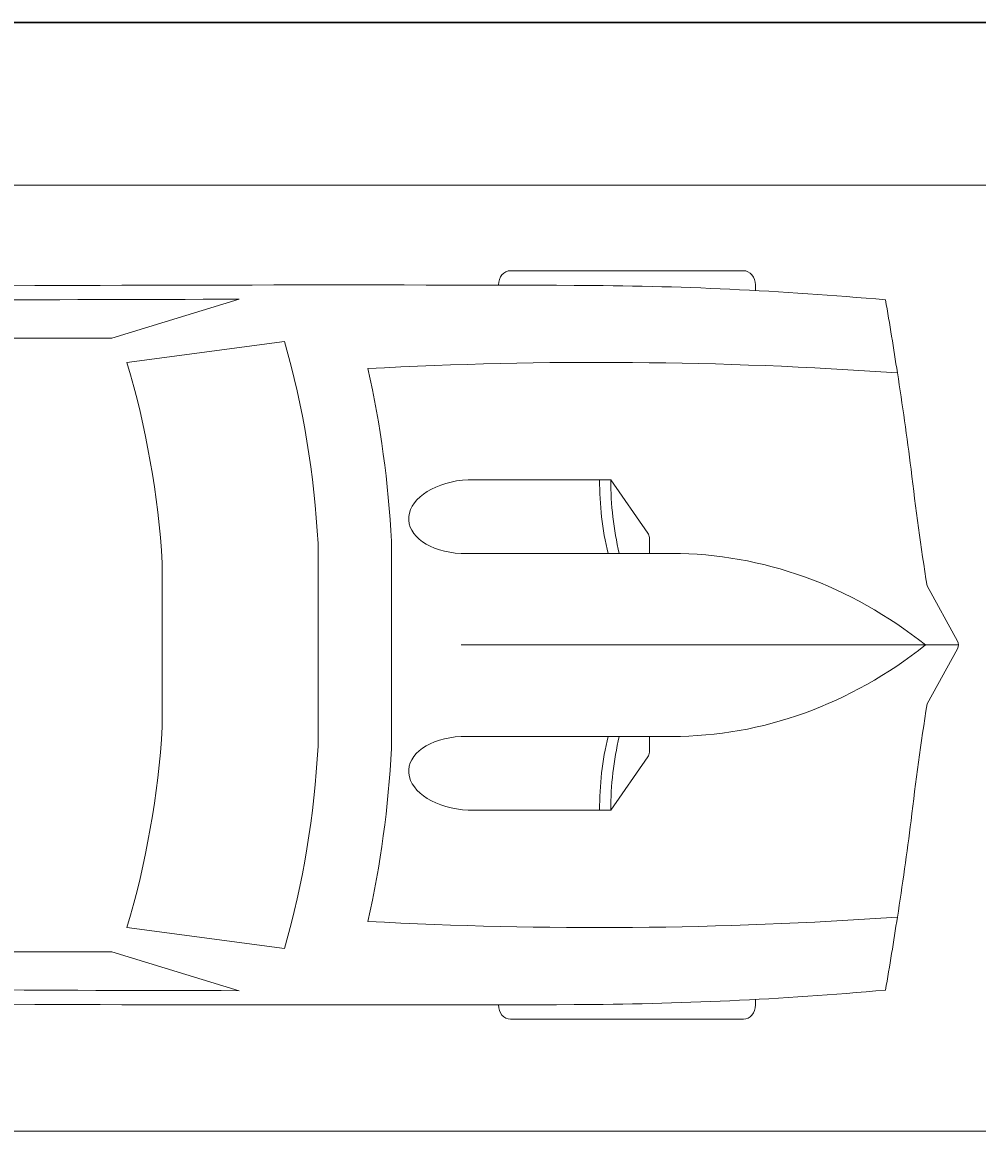
# Model space of a CAD drawing. Units: inches. Extents: x -46 to 1145, y -527 to 760.
# Tile 13 of 57: x 380 to 479, y -157 to -39. Entities that reach past the tile are written whole.
import ezdxf

# ---------------------------------------------------------------- set-up
doc = ezdxf.new("R2010")
doc.units = ezdxf.units.IN
doc.header["$MEASUREMENT"] = 0
for name, color, linetype, lineweight in [('A-ANNO-DIMS', 2, 'Continuous', 18), ('C-PKNG', 8, 'Continuous', 18), ('C-PKNG-VEHI', 8, 'Continuous', 13), ('C-SITE', 7, 'Continuous', 30)]:
    doc.layers.add(name, color=color, linetype=linetype, lineweight=lineweight)
doc.styles.get("Standard").update_dxf_attribs({"font": 'arial.ttf'})
doc.dimstyles.get("Standard").update_dxf_attribs({"dimtxt": 0.18, "dimasz": 0.18, "dimexe": 0.18, "dimexo": 0.0625, "dimgap": 0.09, "dimtad": 0, "dimtih": 1, "dimtoh": 1, "dimdec": 0, "dimzin": 0, "dimdsep": 46, "dimlunit": 3, "dimtxsty": 'Standard', "dimcen": 0.09, "dimadec": 0, "dimazin": 0, "dimtfac": 1, "dimtdec": 0, "dimtofl": 0, "dimtmove": 0, "dimatfit": 3, "dimfxl": 1, "dimtolj": 1, "dimtzin": 0, "dimarcsym": 0})

# ---------------------------------------------------------------- blocks, each defined once
blk = doc.blocks.new('*U640')
for p, q in [((1182.5, 987.8), (567.7, 987.8)), ((3472.1, 987.8), (4086.9, 987.8)), ((536, 950.2), (536, 935.5)), ((1214.1, 949.7), (1214.1, 950.2)), ((3440.5, 941.7), (3440.5, 950.2)), ((4118.5, 950.2), (4118.5, 934.1)), ((2234.8, 809.5), (1898.9, 912.4)), ((3411.6, 904.3), (3029.9, 807.2)), ((4736.4, -850.9), (4736.4, 850.9)), ((4785.3, -832.1), (4785.3, 832.1)), ((1778.8, 801), (2194.7, 745.5)), ((3515.9, 745.5), (3994.1, 745.5)), ((4736.4, 745.5), (4242, 745.5)), ((4178.7, 670.3), (4178.7, -670.3)), ((819.6, 295.3), (917.7, 436.1)), ((917.7, 436.1), (1293.8, 436.1)), ((815.9, 241.4), (815.9, 283.3)), ((1496.5, -273.7), (1496.5, 273.7)), ((756.2, 241.4), (1312.8, 241.4)), ((1690.4, -267.4), (1690.4, 267.4)), ((4736.4, -267.4), (4736.4, 267.4)), ((2101.5, 215.8), (2101.5, -215.8)), ((83, 155.7), (2.6, 10.3)), ((0, 0), (1312.8, 0)), ((2.6, -10.3), (83, -155.7)), ((756.2, -241.4), (1312.8, -241.4)), ((815.9, -241.4), (815.9, -283.3)), ((819.6, -295.3), (917.7, -436.1)), ((917.7, -436.1), (1293.8, -436.1)), ((2194.7, -745.5), (1778.8, -801)), ((3994.1, -745.5), (3515.9, -745.5)), ((4242, -745.5), (4736.4, -745.5)), ((2234.8, -809.5), (1898.9, -912.4)), ((3411.6, -904.3), (3029.9, -807.2)), ((536, -950.2), (536, -935.5)), ((1214.1, -949.7), (1214.1, -950.2)), ((3440.5, -941.7), (3440.5, -950.2)), ((4118.5, -950.2), (4118.5, -934.1)), ((1182.5, -987.8), (567.7, -987.8)), ((3472.1, -987.8), (4086.9, -987.8))]:
    blk.add_line(p, q)
for centre, major_axis, ratio, start_param, end_param in [((567.7, 950.2), (0, -37.6), 0.842304, 3.141593, 4.712389), ((1182.5, 950.2), (0, 37.6), 0.842304, -1.570796, 0), ((3472.1, 950.2), (0, -37.6), 0.842304, 3.141593, 4.712389), ((4086.9, 950.2), (0, 37.6), 0.842304, -1.570796, 0), ((4588, 910.3), (0, 56.4), 0.842304, -0.013017, 1.249894), ((1637.8, -268131.5), (0, 269121), 0.842304, -0.013397, -0.013017), ((4673.1, 832.1), (0, -133.3), 0.842304, 1.570796, 3.128196), ((1046.3, -12467.9), (0, 13417.1), 0.842304, 0.00281, 0.075598), ((1637.8, -268112.7), (0, 269062.9), 0.842304, -0.013397, 0.002797), ((4673.1, 850.9), (0, -75.2), 0.842304, 1.570796, 3.128196), ((6757.2, -699.1), (0, 7958), 0.842304, 1.367076, 1.39176), ((1637.8, -268112.7), (0, -269025.3), 0.842304, 3.133765, 3.140441), ((2433, -93125.4), (0, -93935.2), 0.842304, 3.134049, 3.144098), ((3436.4, 136.8), (0, 2077), 0.842304, 1.245306, 1.50788), ((951.8, -15086.6), (0, -15832.5), 0.842304, 3.096046, 3.200911), ((6583, -699.1), (0, -7754.7), 0.842304, 4.528606, 4.561838), ((3413.8, 136.8), (0, -2280.3), 0.842304, 4.449482, 4.652344), ((3799.7, 71.1), (0, -2021.3), 0.842304, 4.372215, 4.640744), ((433.9, 0), (0, 3734.3), 0.842304, 4.511394, 4.913384), ((912, 0), (0, 3734.3), 0.842304, 4.511394, 4.913384), ((4242, 670.3), (0, 75.2), 0.842304, 0, 1.570796), ((-5194.2, 1330.9), (0, -6374.4), 0.842304, 1.385369, 1.434372), ((331.1, 432), (0, 696.4), 0.842304, 4.435146, 4.718221), ((360.7, 432), (0, 696.4), 0.842304, 4.435146, 4.718221), ((1290.1, 338.8), (161, -9.1), 0.603834, -1.395552, 1.581315), ((831.8, 283.3), (0, 18.8), 0.842304, 0.879714, 1.570796), ((756.2, -1185.2), (0, 1426.7), 0.842304, 0, 0.590319), ((15.8, 0), (0, -18.8), 0.842304, 4.131459, 5.293319), ((756.2, 1185.2), (0, 1426.7), 0.842304, 2.551274, 3.141593), ((-5194.2, -1330.9), (0, 6374.4), 0.842304, -1.434372, -1.385369), ((3799.7, -71.1), (0, -2021.3), 0.842304, -1.499151, -1.230623), ((331.1, -432), (0, -696.4), 0.842304, 1.564964, 1.848039), ((360.7, -432), (0, -696.4), 0.842304, 1.564964, 1.848039), ((3436.4, -136.8), (0, -2077), 0.842304, -1.50788, -1.245306), ((831.8, -283.3), (0, -18.8), 0.842304, 4.712389, 5.403472), ((3413.8, -136.8), (0, -2280.3), 0.842304, -1.510751, -1.307889), ((6583, 699.1), (0, 7754.7), 0.842304, 1.721348, 1.754579), ((4242, -670.3), (0, -75.2), 0.842304, 4.712389, 6.283185), ((6757.2, 699.1), (0, 7958), 0.842304, 1.749832, 1.774517), ((951.8, 15086.6), (0, -15832.5), 0.842304, -0.059319, 0.045547), ((2433, 93125.4), (0, -93935.2), 0.842304, -0.002505, 0.007544), ((4673.1, -832.1), (0, -133.3), 0.842304, 0.013397, 1.570796), ((4673.1, -850.9), (0, 75.2), 0.842304, 3.15499, 4.712389), ((1046.3, 12467.9), (0, -13417.1), 0.842304, -0.075598, -0.00281), ((1637.8, 268112.7), (0, -269025.3), 0.842304, 0.001152, 0.007828), ((567.7, -950.2), (0, 37.6), 0.842304, 1.570796, 3.141593), ((1637.8, 268112.7), (0, 269062.9), 0.842304, 3.138796, 3.15499), ((1182.5, -950.2), (0, -37.6), 0.842304, 0, 1.570796), ((3472.1, -950.2), (0, -37.6), 0.842304, -1.570796, 0), ((4086.9, -950.2), (0, 37.6), 0.842304, 3.141593, 4.712389), ((4588, -910.3), (0, -56.4), 0.842304, -1.249894, 0.013017), ((1637.8, 268131.5), (0, 269121), 0.842304, 3.15461, 3.15499)]:
    blk.add_ellipse(centre, major_axis=major_axis, ratio=ratio, start_param=start_param, end_param=end_param)
at = {"extrusion": (0, 0, -1)}
blk.add_ellipse((1290.1, -338.8), major_axis=(161, 9.1), ratio=0.603834, start_param=-1.395552, end_param=1.581315, dxfattribs=at)
blk = doc.blocks.new('*D702')
at = {"layer": 'A-ANNO-DIMS', "color": 0, "lineweight": -2, "transparency": 16777216}
for p, q in [((189.63, -39.48), (1145.34, -39.48)), ((1145.16, -39.66), (1145.16, -249.3)), ((1145.16, -459.3), (1145.16, -249.66)), ((183.63, -459.48), (1145.34, -459.48))]:
    blk.add_line(p, q, dxfattribs=at)
at = {"layer": 'A-ANNO-DIMS', "color": 0, "transparency": 16777216}
for points in [[(1145.13, -39.66), (1145.19, -39.66), (1145.16, -39.48)], [(1145.13, -459.3), (1145.19, -459.3), (1145.16, -459.48)]]:
    blk.add_solid(points, dxfattribs=at)
at = {"layer": 'Defpoints', "color": 0, "transparency": 16777216}
for p in [(189.56, -39.48), (1145.16, -39.48), (183.56, -459.48)]:
    blk.add_point(p, dxfattribs=at)
at = {"layer": 'A-ANNO-DIMS', "color": 0, "transparency": 16777216, "insert": (1145.16, -249.48), "char_height": 0.18, "attachment_point": 5}
blk.add_mtext('\\A1;420', dxfattribs=at)

msp = doc.modelspace()

# ---------------------------------------------------------------- linework, layer by layer
at = {"layer": 'C-PKNG'}
msp.add_lwpolyline([(501.7297, -154.6684), (273.5156, -154.6684), (273.5156, -56.3706), (501.7297, -56.3706)], close=True, dxfattribs=at)
at = {"layer": 'C-SITE'}
msp.add_line((590.0637, -39.4824), (189.5637, -39.4824), dxfattribs=at)

# ---------------------------------------------------------------- block references
at = {"layer": 'C-PKNG-VEHI', "xscale": 0.0393700787401575, "yscale": 0.0393700787401575, "zscale": 0.0393700787401575, "rotation": 180}
msp.add_blockref('*U640', (476.808, -104.1506), dxfattribs=at)

# ---------------------------------------------------------------- dimensions: what is measured, and where the dimension line sits
at = {"layer": 'A-ANNO-DIMS'}
dim = msp.add_linear_dim(base=(1145.1637, -39.4824), p1=(183.5637, -459.4824), p2=(189.5637, -39.4824), angle=90, dimstyle='Standard', override={"dimdec": 0, "dimlfac": 1, "dimrnd": 0, "dimzin": 0, "dimdsep": 46, "dimlunit": 2}, dxfattribs=at)
dim.commit()
dim.dimension.update_dxf_attribs({"geometry": '*D702', "text_midpoint": (1145.1637, -249.4824)})

doc.saveas('drawing.dxf')
